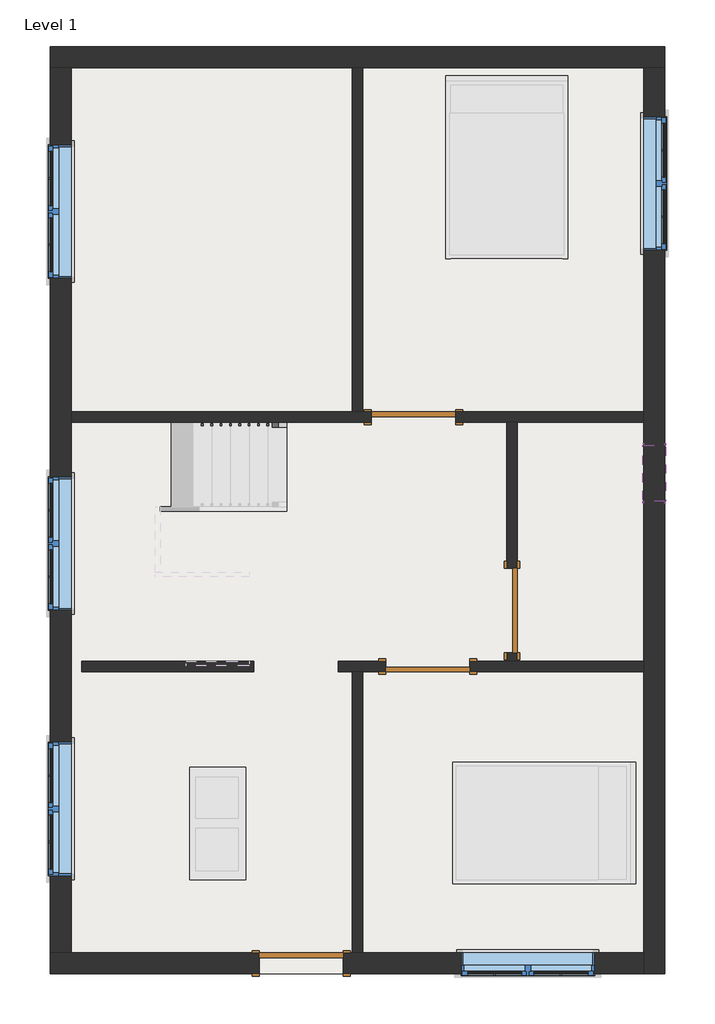
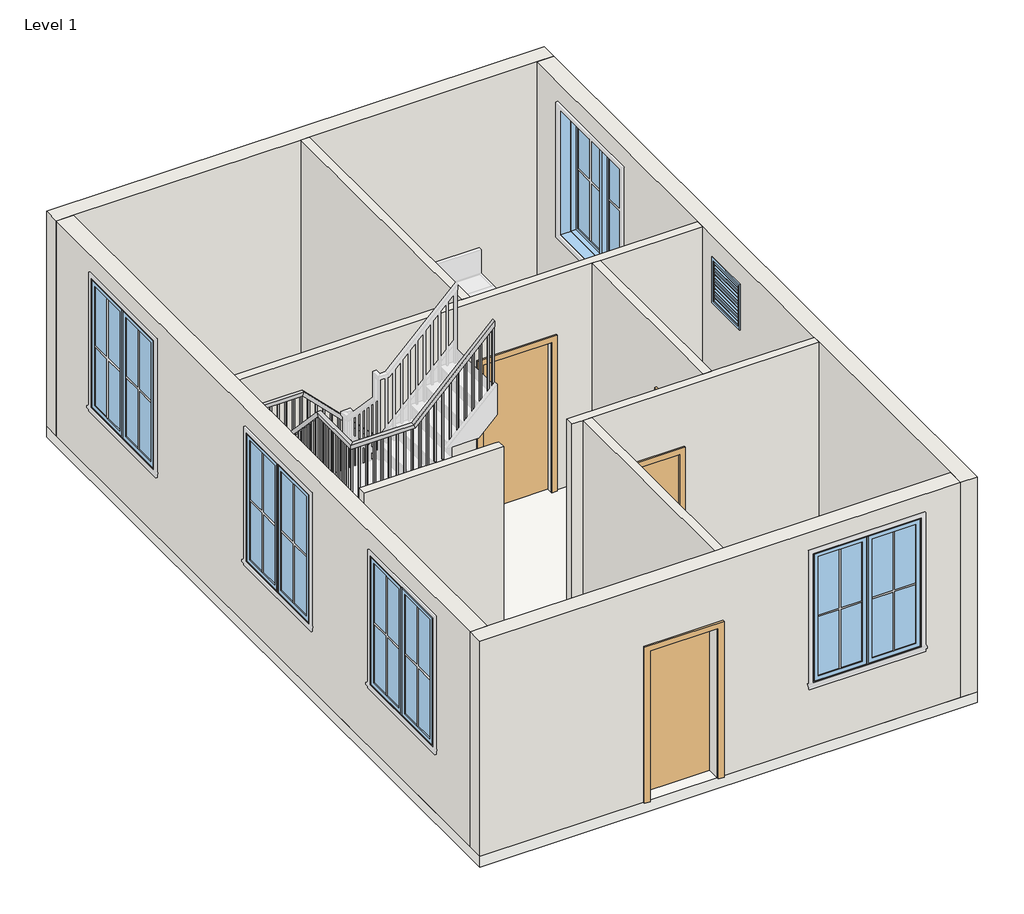
# One storey, part 1 of 2: 10 walls, 6 windows, 4 doors, 1 railing, 1 slab.
"""IFC4 building model written with IfcOpenShell, lengths in millimetres."""

from ifc_helpers import new_model, si_unit, frame, origin, origin_with_axes, place, context, project, spatial, polyline, outline, extrude, faceted_brep, transform, mapped, element, save
from components import door_e5f9f3c4, door_0ca8825f, window_9ac97e1a, window_f2d8fef0

model = new_model("IFC4")

# Units and contexts
model_context = context("Model", 3, world=origin())
ifc_project = project(units=[si_unit("LENGTHUNIT", "METRE", prefix="MILLI")], contexts=[model_context])

# Site, building, storey
site = spatial("IfcSite", under=ifc_project)
building = spatial("IfcBuilding", under=site)
storey = spatial("IfcBuildingStorey", under=building, Name="Level 1", Elevation=0.0)

# Doors
placement = place(None, origin())
door_shape = door_e5f9f3c4(model_context)
element("IfcDoor", 1, ObjectType="Single-Flush : 36\" x 84\"", at=placement, inside=storey, context=model_context, shape_type="MappedRepresentation", body=[
    mapped(door_shape, transform((-2225.1840247, 979.1819954, 0.0), x_axis=(1.0, 0.0, 0.0), y_axis=(0.0, 1.0, 0.0), z_axis=(0.0, 0.0, 1.0))),
])
element("IfcDoor", 2, ObjectType="Single-Flush : 36\" x 84\"", at=placement, inside=storey, context=model_context, shape_type="MappedRepresentation", body=[
    mapped(door_shape, transform((-1158.3840247, -1116.3180046, 0.0), x_axis=(0.0, -1.0, 0.0), y_axis=(1.0, 0.0, 0.0), z_axis=(0.0, 0.0, 1.0))),
])
element("IfcDoor", 3, ObjectType="Single-Flush : 36\" x 84\"", at=placement, inside=storey, context=model_context, shape_type="MappedRepresentation", body=[
    mapped(door_shape, transform((-2072.7840247, -1725.9180046, 0.0), x_axis=(-1.0, 0.0, 0.0), y_axis=(0.0, -1.0, 0.0), z_axis=(0.0, 0.0, 1.0))),
])
door_2_shape = door_0ca8825f(model_context)
element("IfcDoor", 4, ObjectType="Single-Flush : 36\" x 84\"", at=placement, inside=storey, context=model_context, shape_type="MappedRepresentation", body=[
    mapped(door_2_shape, transform((-3444.3840247, -4945.3680046, 0.0), x_axis=(1.0, 0.0, 0.0), y_axis=(0.0, 1.0, 0.0), z_axis=(0.0, 0.0, 1.0))),
])

# Railing
element("IfcRailing", 5, ObjectType="Handrail - Rectangular", at=placement, inside=storey, context=model_context, shape_type="SolidModel", body=[
    faceted_brep([(-3603.1340247, 871.2319954, 1117.6), (-3603.1340247, 871.2319954, 1045.757951), (-3603.1340247, 922.0319954, 1045.757951), (-3603.1340247, 922.0319954, 1117.6), (-5097.5006913, 871.2319954, 2611.9666667), (-5118.5427403, 871.2319954, 2561.1666667), (-5118.5427403, 922.0319954, 2561.1666667), (-5097.5006913, 922.0319954, 2611.9666667), (-5889.1340247, 871.2319954, 2611.9666667), (-5889.1340247, 871.2319954, 2561.1666667), (-5939.9340247, 922.0319954, 2561.1666667), (-5939.9340247, 922.0319954, 2611.9666667), (-5889.1340247, 130.6632454, 2611.9666667), (-5889.1340247, 108.6550591, 2561.1666667), (-5939.9340247, 108.6550591, 2561.1666667), (-5939.9340247, 130.6632454, 2611.9666667), (-5889.1340247, -877.3992546, 3687.2333333), (-5889.1340247, -899.4074409, 3636.4333333), (-5939.9340247, -899.4074409, 3636.4333333), (-5939.9340247, -877.3992546, 3687.2333333), (-5889.1340247, -1617.9680046, 3687.2333333), (-5889.1340247, -1617.9680046, 3636.4333333), (-5939.9340247, -1668.7680046, 3636.4333333), (-5939.9340247, -1668.7680046, 3687.2333333), (-5097.5006913, -1617.9680046, 3687.2333333), (-5076.4586424, -1617.9680046, 3636.4333333), (-5076.4586424, -1668.7680046, 3636.4333333), (-5097.5006913, -1668.7680046, 3687.2333333), (-4009.5340247, -1617.9680046, 4775.2), (-4009.5340247, -1668.7680046, 4775.2), (-4009.5340247, -1668.7680046, 4703.357951), (-4009.5340247, -1617.9680046, 4703.357951)], [[[0, 1, 2, 3]], [[1, 0, 4, 5]], [[2, 1, 5, 6]], [[3, 2, 6, 7]], [[0, 3, 7, 4]], [[5, 4, 8, 9]], [[6, 5, 9, 10]], [[7, 6, 10, 11]], [[4, 7, 11, 8]], [[9, 8, 12, 13]], [[10, 9, 13, 14]], [[11, 10, 14, 15]], [[8, 11, 15, 12]], [[13, 12, 16, 17]], [[14, 13, 17, 18]], [[15, 14, 18, 19]], [[12, 15, 19, 16]], [[17, 16, 20, 21]], [[18, 17, 21, 22]], [[19, 18, 22, 23]], [[16, 19, 23, 20]], [[21, 20, 24, 25]], [[22, 21, 25, 26]], [[23, 22, 26, 27]], [[20, 23, 27, 24]], [[28, 29, 30, 31]], [[25, 24, 28, 31]], [[26, 25, 31, 30]], [[27, 26, 30, 29]], [[24, 27, 29, 28]]]),
    extrude(outline(polyline([(4636.682951, -4076.2090247), (4617.632951, -4095.2590247), (3657.6, -4095.2590247), (3657.6, -4076.2090247), (4636.682951, -4076.2090247)])), frame((0.0, -1652.8930046, 0.0), z_axis=(0.0, 1.0, 0.0), x_axis=(0.0, 0.0, 1.0)), (0.0, 0.0, 1.0), 19.05),
    extrude(outline(polyline([(4535.082951, -4177.8090247), (4516.032951, -4196.8590247), (3657.6, -4196.8590247), (3657.6, -4177.8090247), (4535.082951, -4177.8090247)])), frame((0.0, -1652.8930046, 0.0), z_axis=(0.0, 1.0, 0.0), x_axis=(0.0, 0.0, 1.0)), (0.0, 0.0, 1.0), 19.05),
    extrude(outline(polyline([(4433.482951, -4279.4090247), (4414.432951, -4298.4590247), (3454.4, -4298.4590247), (3454.4, -4279.4090247), (4433.482951, -4279.4090247)])), frame((0.0, -1652.8930046, 0.0), z_axis=(0.0, 1.0, 0.0), x_axis=(0.0, 0.0, 1.0)), (0.0, 0.0, 1.0), 19.05),
    extrude(outline(polyline([(4331.882951, -4381.0090247), (4312.832951, -4400.0590247), (3454.4, -4400.0590247), (3454.4, -4381.0090247), (4331.882951, -4381.0090247)])), frame((0.0, -1652.8930046, 0.0), z_axis=(0.0, 1.0, 0.0), x_axis=(0.0, 0.0, 1.0)), (0.0, 0.0, 1.0), 19.05),
    extrude(outline(polyline([(4230.282951, -4482.6090247), (4211.232951, -4501.6590247), (3251.2, -4501.6590247), (3251.2, -4482.6090247), (4230.282951, -4482.6090247)])), frame((0.0, -1652.8930046, 0.0), z_axis=(0.0, 1.0, 0.0), x_axis=(0.0, 0.0, 1.0)), (0.0, 0.0, 1.0), 19.05),
    extrude(outline(polyline([(4128.682951, -4584.2090247), (4109.632951, -4603.2590247), (3251.2, -4603.2590247), (3251.2, -4584.2090247), (4128.682951, -4584.2090247)])), frame((0.0, -1652.8930046, 0.0), z_axis=(0.0, 1.0, 0.0), x_axis=(0.0, 0.0, 1.0)), (0.0, 0.0, 1.0), 19.05),
    extrude(outline(polyline([(4027.082951, -4685.8090247), (4008.032951, -4704.8590247), (3048.0, -4704.8590247), (3048.0, -4685.8090247), (4027.082951, -4685.8090247)])), frame((0.0, -1652.8930046, 0.0), z_axis=(0.0, 1.0, 0.0), x_axis=(0.0, 0.0, 1.0)), (0.0, 0.0, 1.0), 19.05),
    extrude(outline(polyline([(3925.482951, -4787.4090247), (3906.432951, -4806.4590247), (3048.0, -4806.4590247), (3048.0, -4787.4090247), (3925.482951, -4787.4090247)])), frame((0.0, -1652.8930046, 0.0), z_axis=(0.0, 1.0, 0.0), x_axis=(0.0, 0.0, 1.0)), (0.0, 0.0, 1.0), 19.05),
    extrude(outline(polyline([(3823.882951, -4889.0090247), (3804.832951, -4908.0590247), (2844.8, -4908.0590247), (2844.8, -4889.0090247), (3823.882951, -4889.0090247)])), frame((0.0, -1652.8930046, 0.0), z_axis=(0.0, 1.0, 0.0), x_axis=(0.0, 0.0, 1.0)), (0.0, 0.0, 1.0), 19.05),
    extrude(outline(polyline([(3722.282951, -4990.6090247), (3703.232951, -5009.6590247), (2844.8, -5009.6590247), (2844.8, -4990.6090247), (3722.282951, -4990.6090247)])), frame((0.0, -1652.8930046, 0.0), z_axis=(0.0, 1.0, 0.0), x_axis=(0.0, 0.0, 1.0)), (0.0, 0.0, 1.0), 19.05),
    extrude(outline(polyline([(-5111.2590247, -1652.8930046), (-5111.2590247, -1633.8430046), (-5092.2090247, -1633.8430046), (-5092.2090247, -1652.8930046), (-5111.2590247, -1652.8930046)])), frame((0.0, 0.0, 2641.6), z_axis=(0.0, 0.0, 1.0), x_axis=(1.0, 0.0, 0.0)), (0.0, 0.0, 1.0), 994.8333333),
    extrude(outline(polyline([(-5212.8590247, -1652.8930046), (-5212.8590247, -1633.8430046), (-5193.8090247, -1633.8430046), (-5193.8090247, -1652.8930046), (-5212.8590247, -1652.8930046)])), frame((0.0, 0.0, 2641.6), z_axis=(0.0, 0.0, 1.0), x_axis=(1.0, 0.0, 0.0)), (0.0, 0.0, 1.0), 994.8333333),
    extrude(outline(polyline([(-5314.4590247, -1652.8930046), (-5314.4590247, -1633.8430046), (-5295.4090247, -1633.8430046), (-5295.4090247, -1652.8930046), (-5314.4590247, -1652.8930046)])), frame((0.0, 0.0, 2641.6), z_axis=(0.0, 0.0, 1.0), x_axis=(1.0, 0.0, 0.0)), (0.0, 0.0, 1.0), 994.8333333),
    extrude(outline(polyline([(-5416.0590247, -1652.8930046), (-5416.0590247, -1633.8430046), (-5397.0090247, -1633.8430046), (-5397.0090247, -1652.8930046), (-5416.0590247, -1652.8930046)])), frame((0.0, 0.0, 2641.6), z_axis=(0.0, 0.0, 1.0), x_axis=(1.0, 0.0, 0.0)), (0.0, 0.0, 1.0), 994.8333333),
    extrude(outline(polyline([(-5517.6590247, -1652.8930046), (-5517.6590247, -1633.8430046), (-5498.6090247, -1633.8430046), (-5498.6090247, -1652.8930046), (-5517.6590247, -1652.8930046)])), frame((0.0, 0.0, 2641.6), z_axis=(0.0, 0.0, 1.0), x_axis=(1.0, 0.0, 0.0)), (0.0, 0.0, 1.0), 994.8333333),
    extrude(outline(polyline([(-5619.2590247, -1652.8930046), (-5619.2590247, -1633.8430046), (-5600.2090247, -1633.8430046), (-5600.2090247, -1652.8930046), (-5619.2590247, -1652.8930046)])), frame((0.0, 0.0, 2641.6), z_axis=(0.0, 0.0, 1.0), x_axis=(1.0, 0.0, 0.0)), (0.0, 0.0, 1.0), 994.8333333),
    extrude(outline(polyline([(-5720.8590247, -1652.8930046), (-5720.8590247, -1633.8430046), (-5701.8090247, -1633.8430046), (-5701.8090247, -1652.8930046), (-5720.8590247, -1652.8930046)])), frame((0.0, 0.0, 2641.6), z_axis=(0.0, 0.0, 1.0), x_axis=(1.0, 0.0, 0.0)), (0.0, 0.0, 1.0), 994.8333333),
    extrude(outline(polyline([(-5822.4590247, -1652.8930046), (-5822.4590247, -1633.8430046), (-5803.4090247, -1633.8430046), (-5803.4090247, -1652.8930046), (-5822.4590247, -1652.8930046)])), frame((0.0, 0.0, 2641.6), z_axis=(0.0, 0.0, 1.0), x_axis=(1.0, 0.0, 0.0)), (0.0, 0.0, 1.0), 994.8333333),
    extrude(outline(polyline([(-5924.0590247, -1532.2430046), (-5905.0090247, -1532.2430046), (-5905.0090247, -1551.2930046), (-5924.0590247, -1551.2930046), (-5924.0590247, -1532.2430046)])), frame((0.0, 0.0, 2641.6), z_axis=(0.0, 0.0, 1.0), x_axis=(1.0, 0.0, 0.0)), (0.0, 0.0, 1.0), 994.8333333),
    extrude(outline(polyline([(-5924.0590247, -1430.6430046), (-5905.0090247, -1430.6430046), (-5905.0090247, -1449.6930046), (-5924.0590247, -1449.6930046), (-5924.0590247, -1430.6430046)])), frame((0.0, 0.0, 2641.6), z_axis=(0.0, 0.0, 1.0), x_axis=(1.0, 0.0, 0.0)), (0.0, 0.0, 1.0), 994.8333333),
    extrude(outline(polyline([(-5924.0590247, -1329.0430046), (-5905.0090247, -1329.0430046), (-5905.0090247, -1348.0930046), (-5924.0590247, -1348.0930046), (-5924.0590247, -1329.0430046)])), frame((0.0, 0.0, 2641.6), z_axis=(0.0, 0.0, 1.0), x_axis=(1.0, 0.0, 0.0)), (0.0, 0.0, 1.0), 994.8333333),
    extrude(outline(polyline([(-5924.0590247, -1227.4430046), (-5905.0090247, -1227.4430046), (-5905.0090247, -1246.4930046), (-5924.0590247, -1246.4930046), (-5924.0590247, -1227.4430046)])), frame((0.0, 0.0, 2641.6), z_axis=(0.0, 0.0, 1.0), x_axis=(1.0, 0.0, 0.0)), (0.0, 0.0, 1.0), 994.8333333),
    extrude(outline(polyline([(-5924.0590247, -1125.8430046), (-5905.0090247, -1125.8430046), (-5905.0090247, -1144.8930046), (-5924.0590247, -1144.8930046), (-5924.0590247, -1125.8430046)])), frame((0.0, 0.0, 2641.6), z_axis=(0.0, 0.0, 1.0), x_axis=(1.0, 0.0, 0.0)), (0.0, 0.0, 1.0), 994.8333333),
    extrude(outline(polyline([(-5924.0590247, -1024.2430046), (-5905.0090247, -1024.2430046), (-5905.0090247, -1043.2930046), (-5924.0590247, -1043.2930046), (-5924.0590247, -1024.2430046)])), frame((0.0, 0.0, 2641.6), z_axis=(0.0, 0.0, 1.0), x_axis=(1.0, 0.0, 0.0)), (0.0, 0.0, 1.0), 994.8333333),
    extrude(outline(polyline([(-5924.0590247, -922.6430046), (-5905.0090247, -922.6430046), (-5905.0090247, -941.6930046), (-5924.0590247, -941.6930046), (-5924.0590247, -922.6430046)])), frame((0.0, 0.0, 2641.6), z_axis=(0.0, 0.0, 1.0), x_axis=(1.0, 0.0, 0.0)), (0.0, 0.0, 1.0), 994.8333333),
    extrude(outline(polyline([(-840.0930046, 3573.1646014), (-821.0430046, 3552.8446014), (-821.0430046, 2641.6), (-840.0930046, 2641.6), (-840.0930046, 3573.1646014)])), frame((-5924.0590247, 0.0, 0.0), z_axis=(1.0, 0.0, 0.0), x_axis=(0.0, 1.0, 0.0)), (0.0, 0.0, 1.0), 19.05),
    extrude(outline(polyline([(-738.4930046, 3464.791268), (-719.4430046, 3444.471268), (-719.4430046, 2438.4), (-738.4930046, 2438.4), (-738.4930046, 3464.791268)])), frame((-5924.0590247, 0.0, 0.0), z_axis=(1.0, 0.0, 0.0), x_axis=(0.0, 1.0, 0.0)), (0.0, 0.0, 1.0), 19.05),
    extrude(outline(polyline([(-636.8930046, 3356.4179347), (-617.8430046, 3336.0979347), (-617.8430046, 2438.4), (-636.8930046, 2438.4), (-636.8930046, 3356.4179347)])), frame((-5924.0590247, 0.0, 0.0), z_axis=(1.0, 0.0, 0.0), x_axis=(0.0, 1.0, 0.0)), (0.0, 0.0, 1.0), 19.05),
    extrude(outline(polyline([(-535.2930046, 3248.0446014), (-516.2430046, 3227.7246014), (-516.2430046, 2235.2), (-535.2930046, 2235.2), (-535.2930046, 3248.0446014)])), frame((-5924.0590247, 0.0, 0.0), z_axis=(1.0, 0.0, 0.0), x_axis=(0.0, 1.0, 0.0)), (0.0, 0.0, 1.0), 19.05),
    extrude(outline(polyline([(-433.6930046, 3139.671268), (-414.6430046, 3119.351268), (-414.6430046, 2235.2), (-433.6930046, 2235.2), (-433.6930046, 3139.671268)])), frame((-5924.0590247, 0.0, 0.0), z_axis=(1.0, 0.0, 0.0), x_axis=(0.0, 1.0, 0.0)), (0.0, 0.0, 1.0), 19.05),
    extrude(outline(polyline([(-332.0930046, 3031.2979347), (-313.0430046, 3010.9779347), (-313.0430046, 2032.0), (-332.0930046, 2032.0), (-332.0930046, 3031.2979347)])), frame((-5924.0590247, 0.0, 0.0), z_axis=(1.0, 0.0, 0.0), x_axis=(0.0, 1.0, 0.0)), (0.0, 0.0, 1.0), 19.05),
    extrude(outline(polyline([(-230.4930046, 2922.9246014), (-211.4430046, 2902.6046014), (-211.4430046, 2032.0), (-230.4930046, 2032.0), (-230.4930046, 2922.9246014)])), frame((-5924.0590247, 0.0, 0.0), z_axis=(1.0, 0.0, 0.0), x_axis=(0.0, 1.0, 0.0)), (0.0, 0.0, 1.0), 19.05),
    extrude(outline(polyline([(-128.8930046, 2814.551268), (-109.8430046, 2794.231268), (-109.8430046, 1828.8), (-128.8930046, 1828.8), (-128.8930046, 2814.551268)])), frame((-5924.0590247, 0.0, 0.0), z_axis=(1.0, 0.0, 0.0), x_axis=(0.0, 1.0, 0.0)), (0.0, 0.0, 1.0), 19.05),
    extrude(outline(polyline([(-27.2930046, 2706.1779347), (-8.2430046, 2685.8579347), (-8.2430046, 1828.8), (-27.2930046, 1828.8), (-27.2930046, 2706.1779347)])), frame((-5924.0590247, 0.0, 0.0), z_axis=(1.0, 0.0, 0.0), x_axis=(0.0, 1.0, 0.0)), (0.0, 0.0, 1.0), 19.05),
    extrude(outline(polyline([(74.3069954, 2597.8046014), (93.3569954, 2577.4846014), (93.3569954, 1625.6), (74.3069954, 1625.6), (74.3069954, 2597.8046014)])), frame((-5924.0590247, 0.0, 0.0), z_axis=(1.0, 0.0, 0.0), x_axis=(0.0, 1.0, 0.0)), (0.0, 0.0, 1.0), 19.05),
    extrude(outline(polyline([(-5924.0590247, 194.9569954), (-5905.0090247, 194.9569954), (-5905.0090247, 175.9069954), (-5924.0590247, 175.9069954), (-5924.0590247, 194.9569954)])), frame((0.0, 0.0, 1625.6), z_axis=(0.0, 0.0, 1.0), x_axis=(1.0, 0.0, 0.0)), (0.0, 0.0, 1.0), 935.5666667),
    extrude(outline(polyline([(-5924.0590247, 296.5569954), (-5905.0090247, 296.5569954), (-5905.0090247, 277.5069954), (-5924.0590247, 277.5069954), (-5924.0590247, 296.5569954)])), frame((0.0, 0.0, 1625.6), z_axis=(0.0, 0.0, 1.0), x_axis=(1.0, 0.0, 0.0)), (0.0, 0.0, 1.0), 935.5666667),
    extrude(outline(polyline([(-5924.0590247, 398.1569954), (-5905.0090247, 398.1569954), (-5905.0090247, 379.1069954), (-5924.0590247, 379.1069954), (-5924.0590247, 398.1569954)])), frame((0.0, 0.0, 1625.6), z_axis=(0.0, 0.0, 1.0), x_axis=(1.0, 0.0, 0.0)), (0.0, 0.0, 1.0), 935.5666667),
    extrude(outline(polyline([(-5924.0590247, 499.7569954), (-5905.0090247, 499.7569954), (-5905.0090247, 480.7069954), (-5924.0590247, 480.7069954), (-5924.0590247, 499.7569954)])), frame((0.0, 0.0, 1625.6), z_axis=(0.0, 0.0, 1.0), x_axis=(1.0, 0.0, 0.0)), (0.0, 0.0, 1.0), 935.5666667),
    extrude(outline(polyline([(-5924.0590247, 601.3569954), (-5905.0090247, 601.3569954), (-5905.0090247, 582.3069954), (-5924.0590247, 582.3069954), (-5924.0590247, 601.3569954)])), frame((0.0, 0.0, 1625.6), z_axis=(0.0, 0.0, 1.0), x_axis=(1.0, 0.0, 0.0)), (0.0, 0.0, 1.0), 935.5666667),
    extrude(outline(polyline([(-5924.0590247, 702.9569954), (-5905.0090247, 702.9569954), (-5905.0090247, 683.9069954), (-5924.0590247, 683.9069954), (-5924.0590247, 702.9569954)])), frame((0.0, 0.0, 1625.6), z_axis=(0.0, 0.0, 1.0), x_axis=(1.0, 0.0, 0.0)), (0.0, 0.0, 1.0), 935.5666667),
    extrude(outline(polyline([(-5924.0590247, 804.5569954), (-5905.0090247, 804.5569954), (-5905.0090247, 785.5069954), (-5924.0590247, 785.5069954), (-5924.0590247, 804.5569954)])), frame((0.0, 0.0, 1625.6), z_axis=(0.0, 0.0, 1.0), x_axis=(1.0, 0.0, 0.0)), (0.0, 0.0, 1.0), 935.5666667),
    extrude(outline(polyline([(-5828.8090247, 906.1569954), (-5828.8090247, 887.1069954), (-5847.8590247, 887.1069954), (-5847.8590247, 906.1569954), (-5828.8090247, 906.1569954)])), frame((0.0, 0.0, 1625.6), z_axis=(0.0, 0.0, 1.0), x_axis=(1.0, 0.0, 0.0)), (0.0, 0.0, 1.0), 935.5666667),
    extrude(outline(polyline([(-5727.2090247, 906.1569954), (-5727.2090247, 887.1069954), (-5746.2590247, 887.1069954), (-5746.2590247, 906.1569954), (-5727.2090247, 906.1569954)])), frame((0.0, 0.0, 1625.6), z_axis=(0.0, 0.0, 1.0), x_axis=(1.0, 0.0, 0.0)), (0.0, 0.0, 1.0), 935.5666667),
    extrude(outline(polyline([(-5625.6090247, 906.1569954), (-5625.6090247, 887.1069954), (-5644.6590247, 887.1069954), (-5644.6590247, 906.1569954), (-5625.6090247, 906.1569954)])), frame((0.0, 0.0, 1625.6), z_axis=(0.0, 0.0, 1.0), x_axis=(1.0, 0.0, 0.0)), (0.0, 0.0, 1.0), 935.5666667),
    extrude(outline(polyline([(-5524.0090247, 906.1569954), (-5524.0090247, 887.1069954), (-5543.0590247, 887.1069954), (-5543.0590247, 906.1569954), (-5524.0090247, 906.1569954)])), frame((0.0, 0.0, 1625.6), z_axis=(0.0, 0.0, 1.0), x_axis=(1.0, 0.0, 0.0)), (0.0, 0.0, 1.0), 935.5666667),
    extrude(outline(polyline([(-5422.4090247, 906.1569954), (-5422.4090247, 887.1069954), (-5441.4590247, 887.1069954), (-5441.4590247, 906.1569954), (-5422.4090247, 906.1569954)])), frame((0.0, 0.0, 1625.6), z_axis=(0.0, 0.0, 1.0), x_axis=(1.0, 0.0, 0.0)), (0.0, 0.0, 1.0), 935.5666667),
    extrude(outline(polyline([(-5320.8090247, 906.1569954), (-5320.8090247, 887.1069954), (-5339.8590247, 887.1069954), (-5339.8590247, 906.1569954), (-5320.8090247, 906.1569954)])), frame((0.0, 0.0, 1625.6), z_axis=(0.0, 0.0, 1.0), x_axis=(1.0, 0.0, 0.0)), (0.0, 0.0, 1.0), 935.5666667),
    extrude(outline(polyline([(-5219.2090247, 906.1569954), (-5219.2090247, 887.1069954), (-5238.2590247, 887.1069954), (-5238.2590247, 906.1569954), (-5219.2090247, 906.1569954)])), frame((0.0, 0.0, 1625.6), z_axis=(0.0, 0.0, 1.0), x_axis=(1.0, 0.0, 0.0)), (0.0, 0.0, 1.0), 935.5666667),
    extrude(outline(polyline([(-5117.6090247, 906.1569954), (-5117.6090247, 887.1069954), (-5136.6590247, 887.1069954), (-5136.6590247, 906.1569954), (-5117.6090247, 906.1569954)])), frame((0.0, 0.0, 1625.6), z_axis=(0.0, 0.0, 1.0), x_axis=(1.0, 0.0, 0.0)), (0.0, 0.0, 1.0), 935.5666667),
    extrude(outline(polyline([(2458.632951, -5016.0090247), (2477.682951, -5035.0590247), (1625.6, -5035.0590247), (1625.6, -5016.0090247), (2458.632951, -5016.0090247)])), frame((0.0, 887.1069954, 0.0), z_axis=(0.0, 1.0, 0.0), x_axis=(0.0, 0.0, 1.0)), (0.0, 0.0, 1.0), 19.05),
    extrude(outline(polyline([(2357.032951, -4914.4090247), (2376.082951, -4933.4590247), (1422.4, -4933.4590247), (1422.4, -4914.4090247), (2357.032951, -4914.4090247)])), frame((0.0, 887.1069954, 0.0), z_axis=(0.0, 1.0, 0.0), x_axis=(0.0, 0.0, 1.0)), (0.0, 0.0, 1.0), 19.05),
    extrude(outline(polyline([(2255.432951, -4812.8090247), (2274.482951, -4831.8590247), (1422.4, -4831.8590247), (1422.4, -4812.8090247), (2255.432951, -4812.8090247)])), frame((0.0, 887.1069954, 0.0), z_axis=(0.0, 1.0, 0.0), x_axis=(0.0, 0.0, 1.0)), (0.0, 0.0, 1.0), 19.05),
    extrude(outline(polyline([(2153.832951, -4711.2090247), (2172.882951, -4730.2590247), (1219.2, -4730.2590247), (1219.2, -4711.2090247), (2153.832951, -4711.2090247)])), frame((0.0, 887.1069954, 0.0), z_axis=(0.0, 1.0, 0.0), x_axis=(0.0, 0.0, 1.0)), (0.0, 0.0, 1.0), 19.05),
    extrude(outline(polyline([(2052.232951, -4609.6090247), (2071.282951, -4628.6590247), (1219.2, -4628.6590247), (1219.2, -4609.6090247), (2052.232951, -4609.6090247)])), frame((0.0, 887.1069954, 0.0), z_axis=(0.0, 1.0, 0.0), x_axis=(0.0, 0.0, 1.0)), (0.0, 0.0, 1.0), 19.05),
    extrude(outline(polyline([(1950.632951, -4508.0090247), (1969.682951, -4527.0590247), (1016.0, -4527.0590247), (1016.0, -4508.0090247), (1950.632951, -4508.0090247)])), frame((0.0, 887.1069954, 0.0), z_axis=(0.0, 1.0, 0.0), x_axis=(0.0, 0.0, 1.0)), (0.0, 0.0, 1.0), 19.05),
    extrude(outline(polyline([(1849.032951, -4406.4090247), (1868.082951, -4425.4590247), (1016.0, -4425.4590247), (1016.0, -4406.4090247), (1849.032951, -4406.4090247)])), frame((0.0, 887.1069954, 0.0), z_axis=(0.0, 1.0, 0.0), x_axis=(0.0, 0.0, 1.0)), (0.0, 0.0, 1.0), 19.05),
    extrude(outline(polyline([(1747.432951, -4304.8090247), (1766.482951, -4323.8590247), (812.8, -4323.8590247), (812.8, -4304.8090247), (1747.432951, -4304.8090247)])), frame((0.0, 887.1069954, 0.0), z_axis=(0.0, 1.0, 0.0), x_axis=(0.0, 0.0, 1.0)), (0.0, 0.0, 1.0), 19.05),
    extrude(outline(polyline([(1645.832951, -4203.2090247), (1664.882951, -4222.2590247), (812.8, -4222.2590247), (812.8, -4203.2090247), (1645.832951, -4203.2090247)])), frame((0.0, 887.1069954, 0.0), z_axis=(0.0, 1.0, 0.0), x_axis=(0.0, 0.0, 1.0)), (0.0, 0.0, 1.0), 19.05),
    extrude(outline(polyline([(1544.232951, -4101.6090247), (1563.282951, -4120.6590247), (609.6, -4120.6590247), (609.6, -4101.6090247), (1544.232951, -4101.6090247)])), frame((0.0, 887.1069954, 0.0), z_axis=(0.0, 1.0, 0.0), x_axis=(0.0, 0.0, 1.0)), (0.0, 0.0, 1.0), 19.05),
    extrude(outline(polyline([(1442.632951, -4000.0090247), (1461.682951, -4019.0590247), (609.6, -4019.0590247), (609.6, -4000.0090247), (1442.632951, -4000.0090247)])), frame((0.0, 887.1069954, 0.0), z_axis=(0.0, 1.0, 0.0), x_axis=(0.0, 0.0, 1.0)), (0.0, 0.0, 1.0), 19.05),
    extrude(outline(polyline([(1341.032951, -3898.4090247), (1360.082951, -3917.4590247), (406.4, -3917.4590247), (406.4, -3898.4090247), (1341.032951, -3898.4090247)])), frame((0.0, 887.1069954, 0.0), z_axis=(0.0, 1.0, 0.0), x_axis=(0.0, 0.0, 1.0)), (0.0, 0.0, 1.0), 19.05),
    extrude(outline(polyline([(1239.432951, -3796.8090247), (1258.482951, -3815.8590247), (406.4, -3815.8590247), (406.4, -3796.8090247), (1239.432951, -3796.8090247)])), frame((0.0, 887.1069954, 0.0), z_axis=(0.0, 1.0, 0.0), x_axis=(0.0, 0.0, 1.0)), (0.0, 0.0, 1.0), 19.05),
    extrude(outline(polyline([(1137.832951, -3695.2090247), (1156.882951, -3714.2590247), (203.2, -3714.2590247), (203.2, -3695.2090247), (1137.832951, -3695.2090247)])), frame((0.0, 887.1069954, 0.0), z_axis=(0.0, 1.0, 0.0), x_axis=(0.0, 0.0, 1.0)), (0.0, 0.0, 1.0), 19.05),
    extrude(outline(polyline([(-5924.0590247, -1633.8430046), (-5905.0090247, -1633.8430046), (-5905.0090247, -1652.8930046), (-5924.0590247, -1652.8930046), (-5924.0590247, -1633.8430046)])), frame((0.0, 0.0, 2641.6), z_axis=(0.0, 0.0, 1.0), x_axis=(1.0, 0.0, 0.0)), (0.0, 0.0, 1.0), 994.8333333),
    extrude(outline(polyline([(-5905.0090247, 906.1569954), (-5905.0090247, 887.1069954), (-5924.0590247, 887.1069954), (-5924.0590247, 906.1569954), (-5905.0090247, 906.1569954)])), frame((0.0, 0.0, 1625.6), z_axis=(0.0, 0.0, 1.0), x_axis=(1.0, 0.0, 0.0)), (0.0, 0.0, 1.0), 935.5666667),
    extrude(outline(polyline([(4703.357951, -4009.5340247), (4684.307951, -4028.5840247), (3657.6, -4028.5840247), (3657.6, -4009.5340247), (4703.357951, -4009.5340247)])), frame((0.0, -1652.8930046, 0.0), z_axis=(0.0, 1.0, 0.0), x_axis=(0.0, 0.0, 1.0)), (0.0, 0.0, 1.0), 19.05),
    extrude(outline(polyline([(1045.757951, -3603.1340247), (1064.807951, -3622.1840247), (203.2, -3622.1840247), (203.2, -3603.1340247), (1045.757951, -3603.1340247)])), frame((0.0, 887.1069954, 0.0), z_axis=(0.0, 1.0, 0.0), x_axis=(0.0, 0.0, 1.0)), (0.0, 0.0, 1.0), 19.05),
])

# Slab
element("IfcSlab", 6, ObjectType="FLOOR 6\"", at=placement, inside=storey, context=model_context, shape_type="SweptSolid", body=[
    extrude(outline(polyline([(498.9659753, 4998.7319954), (498.9659753, -5059.6680046), (-6168.5340247, -5059.6680046), (-6168.5340247, 4998.7319954), (498.9659753, 4998.7319954)])), frame((0.0, 0.0, -152.4), z_axis=(0.0, 0.0, 1.0), x_axis=(1.0, 0.0, 0.0)), (0.0, 0.0, 1.0), 152.4),
])

# Walls
element("IfcWall", 7, ObjectType="WALL 4.5\"", at=placement, inside=storey, context=model_context, shape_type="SweptSolid", body=[
    extrude(outline(polyline([(-2891.9340247, 1036.3319954), (-2891.9340247, 4770.1319954), (-2777.6340247, 4770.1319954), (-2777.6340247, 1036.3319954), (-2891.9340247, 1036.3319954)])), origin_with_axes(), (0.0, 0.0, 1.0), 3048.0),
])
element("IfcWall", 8, ObjectType="WALL 4.5\"", at=placement, inside=storey, context=model_context, shape_type="Brep", body=[
    faceted_brep([(-1767.9840247, 922.0319954, 2133.6), (-1767.9840247, 922.0319954, 0.0), (-1215.5340247, 922.0319954, 0.0), (-1101.2340247, 922.0319954, 0.0), (270.3659753, 922.0319954, 0.0), (270.3659753, 922.0319954, 3048.0), (-1101.2340247, 922.0319954, 3048.0), (-1215.5340247, 922.0319954, 3048.0), (-3552.3340247, 922.0319954, 3048.0), (-5889.1340247, 922.0319954, 3048.0), (-5939.9340247, 922.0319954, 3048.0), (-5939.9340247, 922.0319954, 0.0), (-2682.3840247, 922.0319954, 0.0), (-2682.3840247, 922.0319954, 2133.6), (270.3659753, 1036.3319954, 0.0), (-1767.9840247, 1036.3319954, 0.0), (-1767.9840247, 1036.3319954, 2133.6), (-2682.3840247, 1036.3319954, 2133.6), (-2682.3840247, 1036.3319954, 0.0), (-2777.6340247, 1036.3319954, 0.0), (-2891.9340247, 1036.3319954, 0.0), (-5939.9340247, 1036.3319954, 0.0), (-5939.9340247, 1036.3319954, 3048.0), (-2891.9340247, 1036.3319954, 3048.0), (-2777.6340247, 1036.3319954, 3048.0), (270.3659753, 1036.3319954, 3048.0)], [[[0, 1, 2, 3, 4, 5, 6, 7, 8, 9, 10, 11, 12, 13]], [[14, 15, 16, 17, 18, 19, 20, 21, 22, 23, 24, 25]], [[12, 11, 21, 20, 19, 18]], [[4, 3, 2, 1, 15, 14]], [[5, 4, 14, 25]], [[11, 10, 22, 21]], [[16, 15, 1, 0]], [[17, 16, 0, 13]], [[18, 17, 13, 12]], [[10, 9, 8, 7, 6, 5, 25, 24, 23, 22]]]),
])
element("IfcWall", 9, ObjectType="WALL 4.5\"", at=placement, inside=storey, context=model_context, shape_type="SweptSolid", body=[
    extrude(outline(polyline([(-1573.5180046, 2133.6), (-1573.5180046, 0.0), (-1668.7680046, 0.0), (-1668.7680046, 3048.0), (922.0319954, 3048.0), (922.0319954, 0.0), (-659.1180046, 0.0), (-659.1180046, 2133.6), (-1573.5180046, 2133.6)])), frame((-1215.5340247, 0.0, 0.0), z_axis=(1.0, 0.0, 0.0), x_axis=(0.0, 1.0, 0.0)), (0.0, 0.0, 1.0), 114.3),
])
element("IfcWall", 10, ObjectType="WALL 4.5\"", at=placement, inside=storey, context=model_context, shape_type="Brep", body=[
    faceted_brep([(-2529.9840247, -1668.7680046, 2133.6), (-2529.9840247, -1668.7680046, 0.0), (-3044.3340247, -1668.7680046, 0.0), (-3044.3340247, -1668.7680046, 3048.0), (-1215.5340247, -1668.7680046, 3048.0), (-1101.2340247, -1668.7680046, 3048.0), (270.3659753, -1668.7680046, 3048.0), (270.3659753, -1668.7680046, 0.0), (-1101.2340247, -1668.7680046, 0.0), (-1215.5340247, -1668.7680046, 0.0), (-1615.5840247, -1668.7680046, 0.0), (-1615.5840247, -1668.7680046, 2133.6), (-3044.3340247, -1783.0680046, 0.0), (-2891.9340247, -1783.0680046, 0.0), (-2777.6340247, -1783.0680046, 0.0), (-2529.9840247, -1783.0680046, 0.0), (-2529.9840247, -1783.0680046, 2133.6), (-1615.5840247, -1783.0680046, 2133.6), (-1615.5840247, -1783.0680046, 0.0), (270.3659753, -1783.0680046, 0.0), (270.3659753, -1783.0680046, 3048.0), (-2777.6340247, -1783.0680046, 3048.0), (-2891.9340247, -1783.0680046, 3048.0), (-3044.3340247, -1783.0680046, 3048.0)], [[[0, 1, 2, 3, 4, 5, 6, 7, 8, 9, 10, 11]], [[12, 13, 14, 15, 16, 17, 18, 19, 20, 21, 22, 23]], [[2, 1, 15, 14, 13, 12]], [[10, 9, 8, 7, 19, 18]], [[3, 2, 12, 23]], [[7, 6, 20, 19]], [[16, 15, 1, 0]], [[17, 16, 0, 11]], [[18, 17, 11, 10]], [[6, 5, 4, 3, 23, 22, 21, 20]]]),
])
element("IfcWall", 11, ObjectType="WALL 4.5\"", at=placement, inside=storey, context=model_context, shape_type="Brep", body=[
    faceted_brep([(-5825.6340247, -1783.0680046, 0.0), (-3958.7340247, -1783.0680046, 0.0), (-3958.7340247, -1783.0680046, 3048.0), (-5825.6340247, -1783.0680046, 3048.0), (-5825.6340247, -1668.7680046, 0.0), (-5825.6340247, -1668.7680046, 3048.0), (-4009.5340247, -1668.7680046, 3048.0), (-3958.7340247, -1668.7680046, 3048.0), (-3958.7340247, -1668.7680046, 0.0)], [[[0, 1, 2, 3]], [[4, 5, 6, 7, 8]], [[1, 0, 4, 8]], [[2, 1, 8, 7]], [[0, 3, 5, 4]], [[3, 2, 7, 6, 5]]]),
])
element("IfcWall", 12, ObjectType="WALL 4.5\"", at=placement, inside=storey, context=model_context, shape_type="SweptSolid", body=[
    extrude(outline(polyline([(-2891.9340247, -4831.0680046), (-2891.9340247, -1783.0680046), (-2777.6340247, -1783.0680046), (-2777.6340247, -4831.0680046), (-2891.9340247, -4831.0680046)])), origin_with_axes(), (0.0, 0.0, 1.0), 3048.0),
])
element("IfcWall", 13, ObjectType="WALL 9\"", at=placement, inside=storey, context=model_context, shape_type="Brep", body=[
    faceted_brep([(-6168.5340247, 4770.1319954, 0.0), (-5939.9340247, 4770.1319954, 0.0), (-2891.9340247, 4770.1319954, 0.0), (-2777.6340247, 4770.1319954, 0.0), (270.3659753, 4770.1319954, 0.0), (498.9659753, 4770.1319954, 0.0), (498.9659753, 4770.1319954, 3048.0), (270.3659753, 4770.1319954, 3048.0), (-2777.6340247, 4770.1319954, 3048.0), (-2891.9340247, 4770.1319954, 3048.0), (-5939.9340247, 4770.1319954, 3048.0), (-6168.5340247, 4770.1319954, 3048.0), (-6168.5340247, 4998.7319954, 0.0), (-6168.5340247, 4998.7319954, 3048.0), (498.9659753, 4998.7319954, 3048.0), (498.9659753, 4998.7319954, 0.0)], [[[0, 1, 2, 3, 4, 5, 6, 7, 8, 9, 10, 11]], [[12, 13, 14, 15]], [[5, 4, 3, 2, 1, 0, 12, 15]], [[6, 5, 15, 14]], [[0, 11, 13, 12]], [[11, 10, 9, 8, 7, 6, 14, 13]]]),
])
element("IfcWall", 14, ObjectType="WALL 9\"", at=placement, inside=storey, context=model_context, shape_type="Brep", body=[
    faceted_brep([(270.3659753, 4770.1319954, 0.0), (270.3659753, 1036.3319954, 0.0), (270.3659753, 922.0319954, 0.0), (270.3659753, -1668.7680046, 0.0), (270.3659753, -1783.0680046, 0.0), (270.3659753, -4831.0680046, 0.0), (270.3659753, -5059.6680046, 0.0), (270.3659753, -5059.6680046, 3048.0), (270.3659753, -4831.0680046, 3048.0), (270.3659753, -1783.0680046, 3048.0), (270.3659753, -1668.7680046, 3048.0), (270.3659753, 922.0319954, 3048.0), (270.3659753, 1036.3319954, 3048.0), (270.3659753, 4770.1319954, 3048.0), (270.3659753, 2788.9319954, 2743.2), (270.3659753, 2788.9319954, 914.4), (270.3659753, 4236.7319954, 914.4), (270.3659753, 4236.7319954, 2743.2), (270.3659753, 64.7819954, 2743.2), (270.3659753, 64.7819954, 2133.6), (270.3659753, 674.3819954, 2133.6), (270.3659753, 674.3819954, 2743.2), (498.9659753, 4770.1319954, 0.0), (498.9659753, 4770.1319954, 3048.0), (498.9659753, -5059.6680046, 3048.0), (498.9659753, -5059.6680046, 0.0), (498.9659753, 2788.9319954, 2743.2), (498.9659753, 4236.7319954, 2743.2), (498.9659753, 4236.7319954, 914.4), (498.9659753, 2788.9319954, 914.4), (498.9659753, 64.7819954, 2743.2), (498.9659753, 674.3819954, 2743.2), (498.9659753, 674.3819954, 2133.6), (498.9659753, 64.7819954, 2133.6)], [[[0, 1, 2, 3, 4, 5, 6, 7, 8, 9, 10, 11, 12, 13], [14, 15, 16, 17], [18, 19, 20, 21]], [[22, 23, 24, 25], [26, 27, 28, 29], [30, 31, 32, 33]], [[6, 5, 4, 3, 2, 1, 0, 22, 25]], [[0, 13, 23, 22]], [[7, 6, 25, 24]], [[15, 14, 26, 29]], [[16, 15, 29, 28]], [[17, 16, 28, 27]], [[14, 17, 27, 26]], [[19, 18, 30, 33]], [[20, 19, 33, 32]], [[21, 20, 32, 31]], [[18, 21, 31, 30]], [[13, 12, 11, 10, 9, 8, 7, 24, 23]]]),
])
element("IfcWall", 15, ObjectType="WALL 9\"", at=placement, inside=storey, context=model_context, shape_type="Brep", body=[
    faceted_brep([(270.3659753, -4831.0680046, 0.0), (-2777.6340247, -4831.0680046, 0.0), (-2891.9340247, -4831.0680046, 0.0), (-2987.1840247, -4831.0680046, 0.0), (-2987.1840247, -4831.0680046, 2133.6), (-3901.5840247, -4831.0680046, 2133.6), (-3901.5840247, -4831.0680046, 0.0), (-5939.9340247, -4831.0680046, 0.0), (-6168.5340247, -4831.0680046, 0.0), (-6168.5340247, -4831.0680046, 3048.0), (-5939.9340247, -4831.0680046, 3048.0), (-2891.9340247, -4831.0680046, 3048.0), (-2777.6340247, -4831.0680046, 3048.0), (270.3659753, -4831.0680046, 3048.0), (-1710.8340247, -4831.0680046, 2743.2), (-1710.8340247, -4831.0680046, 914.4), (-263.0340247, -4831.0680046, 914.4), (-263.0340247, -4831.0680046, 2743.2), (-2987.1840247, -5059.6680046, 2133.6), (-2987.1840247, -5059.6680046, 0.0), (270.3659753, -5059.6680046, 0.0), (270.3659753, -5059.6680046, 3048.0), (-6168.5340247, -5059.6680046, 3048.0), (-6168.5340247, -5059.6680046, 0.0), (-3901.5840247, -5059.6680046, 0.0), (-3901.5840247, -5059.6680046, 2133.6), (-1710.8340247, -5059.6680046, 2743.2), (-263.0340247, -5059.6680046, 2743.2), (-263.0340247, -5059.6680046, 914.4), (-1710.8340247, -5059.6680046, 914.4)], [[[0, 1, 2, 3, 4, 5, 6, 7, 8, 9, 10, 11, 12, 13], [14, 15, 16, 17]], [[18, 19, 20, 21, 22, 23, 24, 25], [26, 27, 28, 29]], [[24, 23, 8, 7, 6]], [[20, 19, 3, 2, 1, 0]], [[0, 13, 21, 20]], [[9, 8, 23, 22]], [[15, 14, 26, 29]], [[16, 15, 29, 28]], [[17, 16, 28, 27]], [[14, 17, 27, 26]], [[4, 3, 19, 18]], [[5, 4, 18, 25]], [[6, 5, 25, 24]], [[13, 12, 11, 10, 9, 22, 21]]]),
])
element("IfcWall", 16, ObjectType="WALL 9\"", at=placement, inside=storey, context=model_context, shape_type="Brep", body=[
    faceted_brep([(-5939.9340247, -4831.0680046, 0.0), (-5939.9340247, 922.0319954, 0.0), (-5939.9340247, 1036.3319954, 0.0), (-5939.9340247, 4770.1319954, 0.0), (-5939.9340247, 4770.1319954, 3048.0), (-5939.9340247, 1036.3319954, 3048.0), (-5939.9340247, 922.0319954, 3048.0), (-5939.9340247, -4831.0680046, 3048.0), (-5939.9340247, -2545.0680046, 2743.2), (-5939.9340247, -2545.0680046, 914.4), (-5939.9340247, -3992.8680046, 914.4), (-5939.9340247, -3992.8680046, 2743.2), (-5939.9340247, 3931.9319954, 2743.2), (-5939.9340247, 3931.9319954, 914.4), (-5939.9340247, 2484.1319954, 914.4), (-5939.9340247, 2484.1319954, 2743.2), (-5939.9340247, 331.4819954, 2743.2), (-5939.9340247, 331.4819954, 914.4), (-5939.9340247, -1116.3180046, 914.4), (-5939.9340247, -1116.3180046, 2743.2), (-6168.5340247, -4831.0680046, 0.0), (-6168.5340247, -4831.0680046, 3048.0), (-6168.5340247, 4770.1319954, 3048.0), (-6168.5340247, 4770.1319954, 0.0), (-6168.5340247, -2545.0680046, 2743.2), (-6168.5340247, -3992.8680046, 2743.2), (-6168.5340247, -3992.8680046, 914.4), (-6168.5340247, -2545.0680046, 914.4), (-6168.5340247, 3931.9319954, 2743.2), (-6168.5340247, 2484.1319954, 2743.2), (-6168.5340247, 2484.1319954, 914.4), (-6168.5340247, 3931.9319954, 914.4), (-6168.5340247, 331.4819954, 2743.2), (-6168.5340247, -1116.3180046, 2743.2), (-6168.5340247, -1116.3180046, 914.4), (-6168.5340247, 331.4819954, 914.4)], [[[0, 1, 2, 3, 4, 5, 6, 7], [8, 9, 10, 11], [12, 13, 14, 15], [16, 17, 18, 19]], [[20, 21, 22, 23], [24, 25, 26, 27], [28, 29, 30, 31], [32, 33, 34, 35]], [[3, 2, 1, 0, 20, 23]], [[0, 7, 21, 20]], [[4, 3, 23, 22]], [[9, 8, 24, 27]], [[10, 9, 27, 26]], [[11, 10, 26, 25]], [[8, 11, 25, 24]], [[13, 12, 28, 31]], [[14, 13, 31, 30]], [[15, 14, 30, 29]], [[12, 15, 29, 28]], [[17, 16, 32, 35]], [[18, 17, 35, 34]], [[19, 18, 34, 33]], [[16, 19, 33, 32]], [[7, 6, 5, 4, 22, 21]]]),
])

# Windows
window_shape = window_9ac97e1a(model_context)
element("IfcWindow", 17, ObjectType="Window-Casement-Double : 57\" x 72\"", at=placement, inside=storey, context=model_context, shape_type="MappedRepresentation", body=[
    mapped(window_shape, transform((-986.9340247, -4945.3680046, 0.0), x_axis=(-1.0, 0.0, 0.0), y_axis=(0.0, -1.0, 0.0), z_axis=(0.0, 0.0, 1.0))),
])
element("IfcWindow", 18, ObjectType="Window-Casement-Double : 57\" x 72\"", at=placement, inside=storey, context=model_context, shape_type="MappedRepresentation", body=[
    mapped(window_shape, transform((-6054.2340247, -3268.9680046, 0.0), x_axis=(0.0, 1.0, 0.0), y_axis=(-1.0, 0.0, 0.0), z_axis=(0.0, 0.0, 1.0))),
])
element("IfcWindow", 19, ObjectType="Window-Casement-Double : 57\" x 72\"", at=placement, inside=storey, context=model_context, shape_type="MappedRepresentation", body=[
    mapped(window_shape, transform((384.6659753, 3512.8319954, 0.0), x_axis=(0.0, -1.0, 0.0), y_axis=(1.0, 0.0, 0.0), z_axis=(0.0, 0.0, 1.0))),
])
element("IfcWindow", 20, ObjectType="Window-Casement-Double : 57\" x 72\"", at=placement, inside=storey, context=model_context, shape_type="MappedRepresentation", body=[
    mapped(window_shape, transform((-6054.2340247, 3208.0319954, 0.0), x_axis=(0.0, 1.0, 0.0), y_axis=(-1.0, 0.0, 0.0), z_axis=(0.0, 0.0, 1.0))),
])
element("IfcWindow", 21, ObjectType="Window-Casement-Double : 57\" x 72\"", at=placement, inside=storey, context=model_context, shape_type="MappedRepresentation", body=[
    mapped(window_shape, transform((-6054.2340247, -392.4180046, 0.0), x_axis=(0.0, 1.0, 0.0), y_axis=(-1.0, 0.0, 0.0), z_axis=(0.0, 0.0, 1.0))),
])
window_2_shape = window_f2d8fef0(model_context)
element("IfcWindow", 22, ObjectType="Window-Louvers : 24\" x 24\"", at=placement, inside=storey, context=model_context, shape_type="MappedRepresentation", body=[
    mapped(window_2_shape, transform((378.3159753, 369.5819954, 1219.2), x_axis=(0.0, 1.0, 0.0), y_axis=(-1.0, 0.0, 0.0), z_axis=(0.0, 0.0, 1.0))),
])

save(model, "model.ifc")

# Revit data of these elements
# Type "Single-Flush : 36\" x 84\""
#   Type Mark = "1"
#   Construction Type Id = "MDOOR"
#   Assembly Code = "C1020"
#   Analytic Construction = "Metal"
#   Thickness = 0' - 2"
#   Heat Transfer Coefficient (U) = 0.651978 BTU/(h·ft²·°F)
#   Height = 7' - 0"
#   Trim Projection Ext = 0' - 1"
#   Trim Projection Int = 0' - 1"
#   Trim Width = 0' - 3"
#   Width = 3' - 0"
#   Define Thermal Properties by = 1
#   Define Thermal Properties by = 1
#   Door Material = Door - Panel
#   Frame Material = Door - Frame
#   Visual Light Transmittance = 0
#   Solar Heat Gain Coefficient = 0
#   Function = (empty or 0)
#   Wall Closure = (empty or 0)
# Type "Handrail - Rectangular"
#   Assembly Code = "C2010400"
#   built-in parameter 1008612 = 0.0416667 (stored number, unit not read)
#   built-in parameter 1008611 = 0.0416667 (stored number, unit not read)
#   built-in parameter 1008609 = 0.333333 (stored number, unit not read)
#   built-in parameter 1008604 = 0.166667 (stored number, unit not read)
#   built-in parameter 1008603 = 0.166667 (stored number, unit not read)
#   Railing Height = 3' - 0"
#   built-in parameter 1008630 = 2
#   built-in parameter 1008610 = 2
#   built-in parameter 1008618 = Baluster - Square : 3/4"
# Type "FLOOR 6\""
#   Assembly Code = "B1010"
#   Function = 0
#   Layers, outside or top first: 0' - 6" no material (function 1)
# Type "WALL 4.5\""
#   Assembly Code = "B2010"
#   Layers, outside or top first: 0' - 4 1/2" no material (function 1)
# Type "WALL 9\""
#   Assembly Code = "B2010"
#   Layers, outside or top first: 0' - 9" no material (function 1)
# Type "Window-Casement-Double : 57\" x 72\""
#   Type Mark = "17"
#   Fire Rating = "0.5h"
#   Assembly Code = "B2020100"
#   Analytic Construction = "Double glazing - domestic"
#   Frame Extension [instance default] = 0' - 0 1/4"
#   Window Inset [instance default] = 0' - 0"
#   Wall Thickness [instance default] = 0' - 6"
#   Interior Wall Closure [instance default] = 0' - 2 1/4"
#   Half Width = 2' - 4 1/2"
#   Visual Light Transmittance = 0.81
#   Thermal Resistance (R) = 1.8146 (h·ft²·°F)/BTU
#   Solar Heat Gain Coefficient = 0.76
#   Rough Width = 4' - 9 1/2"
#   Rough Height = 6' - 0 1/2"
#   Height = 6' - 0"
#   Heat Transfer Coefficient (U) = 0.5511 BTU/(h·ft²·°F)
#   Exterior Wall Closure [instance default] = 0' - 1 1/4"
#   Extension Jamb [instance default] = 0' - 2 1/4"
#   Default Sill Height = 3' - 0"
#   Width = 4' - 9"
#   Define Thermal Properties by = 0
#   Muntin Visibility = yes
#   Interior Trim Visibility [instance default] = yes
#   Exterior Trim Visibility [instance default] = yes
#   Extension Jamb Visibility [instance default] = yes
#   Interior Trim Material = Wood - Stained
#   Muntin Pattern = Muntin Pattern_2x2 : Muntin Pattern_2x2
#   Interior Trim = Trim-Window-Interior-Flat : Picture Frame
#   Interior Frame Material = Wood - Stained
#   Glass Panel Material = Glass
#   Exterior Trim Material = Clad - White
#   Exterior Trim = Trim-Window-Exterior-Flat : with Sill
#   Exterior Frame Material = Clad - White
#   Wall Closure = (empty or 0)
# Type "Window-Louvers : 24\" x 24\""
#   Type Mark = "18"
#   Construction Type Id = "GSP4R"
#   Assembly Code = "B20"
#   Analytic Construction = "1/8 in Pilkington single glazing"
#   Visual Light Transmittance = 0.9
#   Thermal Resistance (R) = 1.53941 (h·ft²·°F)/BTU
#   Solar Heat Gain Coefficient = 0.78
#   Max Height = 1' - 11.74264"
#   Height = 2' - 0"
#   Heat Transfer Coefficient (U) = 0.6496 BTU/(h·ft²·°F)
#   Blade Width [instance default] = 1' - 10 1/2"
#   Blade Vertical Thickness = 0' - 0.35355"
#   Blade Thickness = 0' - 0 1/4"
#   Blade Spacing = 0' - 1 1/2"
#   Blade Height = 0' - 1.85355"
#   Blade Depth = 0' - 3"
#   Blade Angle = 45.00°
#   Default Sill Height = 3' - 0"
#   Trim Projection_Exterior = 0' - 0 1/2"
#   Trim Projection_Interior = 0' - 0 1/2"
#   Trim Width_Exterior = 0' - 1 1/2"
#   Trim Width_Interior = 0' - 1 1/2"
#   Width = 2' - 0"
#   Max Blade Count = 12
#   Define Thermal Properties by = 1
#   Blade Count = 12
#   Frame Material = Birch
#   Louver Material = Birch
#   Trim Exterior Material = Birch
#   Trim Interior Material = Birch
#   Wall Closure = (empty or 0)
# Elements 1, 2, 3, 4 (IfcDoor, "Single-Flush : 36\" x 84\"")
#   Phase Created = New Construction
#   Materials on its faces: "Door - Frame", "Door - Panel"
# Element 5 (IfcRailing, "Handrail - Rectangular")
#   Phase Created = New Construction
# Element 6 (IfcSlab, "FLOOR 6\"")
#   Height Offset From Level = 0' - 0"
#   Phase Created = New Construction
#   Materials on its faces: "Default Floor"
# Elements 7, 8, 9, 10, 11, 12 (IfcWall, "WALL 4.5\"")
#   Top Offset = 0' - 0"
#   Base Offset = 0' - 0"
#   Unconnected Height = 10' - 0"
#   wall height = 10' - 0"
#   Phase Created = New Construction
#   Base Constraint = Level 1
#   Materials on its faces: "Default Wall"
# Elements 13, 14, 15, 16 (IfcWall, "WALL 9\"")
#   Top Offset = 0' - 0"
#   Base Offset = 0' - 0"
#   Unconnected Height = 10' - 0"
#   wall height = 10' - 0"
#   Phase Created = New Construction
#   Base Constraint = Level 1
#   Materials on its faces: "Default Wall", "Parking Stripe"
# Element 17 (IfcWindow, "Window-Casement-Double : 57\" x 72\"")
#   Mark = "1"
#   Window Inset = 0' - 0"
#   Interior Wall Closure = 0' - 2 1/4"
#   Frame Extension = 0' - 0 1/4"
#   Exterior Wall Closure = 0' - 1 1/4"
#   Interior Trim Visibility = yes
#   Exterior Trim Visibility = yes
#   Phase Created = New Construction
#   Materials on its faces: "Wood - Stained", "Glass", "Clad - White"
# Element 18 (IfcWindow, "Window-Casement-Double : 57\" x 72\"")
#   Mark = "2"
#   Window Inset = 0' - 0"
#   Interior Wall Closure = 0' - 2 1/4"
#   Frame Extension = 0' - 0 1/4"
#   Exterior Wall Closure = 0' - 1 1/4"
#   Interior Trim Visibility = yes
#   Exterior Trim Visibility = yes
#   Phase Created = New Construction
#   Materials on its faces: "Wood - Stained", "Glass", "Clad - White"
# Element 19 (IfcWindow, "Window-Casement-Double : 57\" x 72\"")
#   Mark = "3"
#   Window Inset = 0' - 0"
#   Interior Wall Closure = 0' - 2 1/4"
#   Frame Extension = 0' - 0 1/4"
#   Exterior Wall Closure = 0' - 1 1/4"
#   Interior Trim Visibility = yes
#   Exterior Trim Visibility = yes
#   Phase Created = New Construction
#   Materials on its faces: "Wood - Stained", "Glass", "Clad - White"
# Element 20 (IfcWindow, "Window-Casement-Double : 57\" x 72\"")
#   Mark = "4"
#   Window Inset = 0' - 0"
#   Interior Wall Closure = 0' - 2 1/4"
#   Frame Extension = 0' - 0 1/4"
#   Exterior Wall Closure = 0' - 1 1/4"
#   Interior Trim Visibility = yes
#   Exterior Trim Visibility = yes
#   Phase Created = New Construction
#   Materials on its faces: "Wood - Stained", "Glass", "Clad - White"
# Element 21 (IfcWindow, "Window-Casement-Double : 57\" x 72\"")
#   Mark = "5"
#   Window Inset = 0' - 0"
#   Interior Wall Closure = 0' - 2 1/4"
#   Frame Extension = 0' - 0 1/4"
#   Exterior Wall Closure = 0' - 1 1/4"
#   Interior Trim Visibility = yes
#   Exterior Trim Visibility = yes
#   Phase Created = New Construction
#   Materials on its faces: "Wood - Stained", "Glass", "Clad - White"
# Element 22 (IfcWindow, "Window-Louvers : 24\" x 24\"")
#   Mark = "6"
#   Blade Width = 1' - 10 1/2"
#   Phase Created = New Construction
#   Materials on its faces: "Birch"
# Materials
#   "Door - Panel": class "Wood", colour RGB 210 159 95, transparency 0, Cost = 0
#   "Door - Frame": colour RGB 118 70 51, transparency 0, Cost = 0
#   "Wood - Stained": class "Wood", colour RGB 224 178 126, transparency 0, Cost = 0
#   "Glass": class "Glass", colour RGB 0 128 192, transparency 0.75, Description = "Soda Lime Glass", Cost = 0
#   "Clad - White": class "Wood", colour RGB 242 242 238, transparency 0, Cost = 0
#   "Birch": class "Wood", colour RGB 224 178 126, transparency 0, Description = "Betula Alleghaniensis", Cost = 0
#   "Default Floor": colour RGB 128 128 128, transparency 0, Cost = 0
#   "Default Wall": colour RGB 128 128 128, transparency 0, Cost = 0
#   "Parking Stripe": class "Paint", colour RGB 250 250 91, transparency 0, Cost = 0
